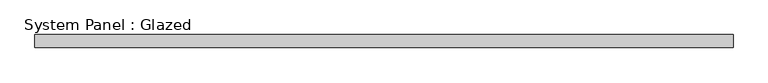
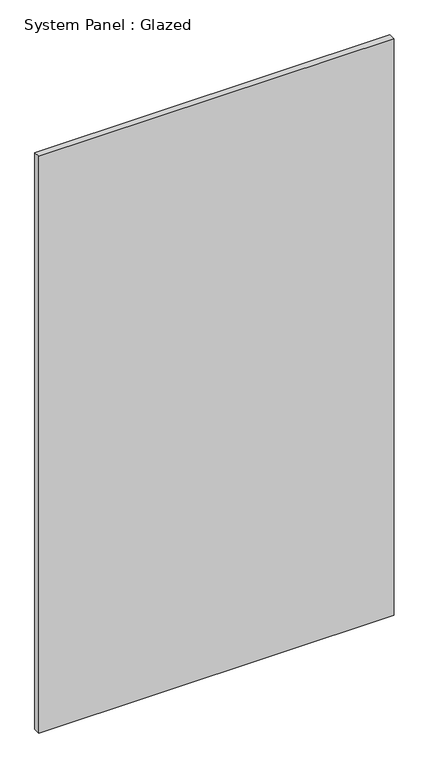
"""IFC4 building model written with IfcOpenShell, lengths in millimetres: plate geometry, System Panel : Glazed."""

from ifc_helpers import new_model, si_unit, origin, origin_with_axes, place, context, project, spatial, polyline, outline, extrude, source, transform, mapped, element, save


def system_panel_glazed_660e552d(model_context):
    return source(origin(), model_context, "Body", "SweptSolid", [
        extrude(outline(polyline([(683.0342567, 19.05), (-683.0342567, 19.05), (-683.0342567, 44.45), (683.0342567, 44.45), (683.0342567, 19.05)])), origin_with_axes(), (0.0, 0.0, 1.0), 2343.15),
    ])


if __name__ == "__main__":
    model = new_model("IFC4")
    model_context = context("Model", 3, world=origin())
    ifc_project = project(units=[si_unit("LENGTHUNIT", "METRE", prefix="MILLI")], contexts=[model_context])
    site = spatial("IfcSite", under=ifc_project)
    building = spatial("IfcBuilding", under=site)
    placement = place(None, origin())
    system_panel_glazed_shape = system_panel_glazed_660e552d(model_context)
    element("IfcPlate", 1, ObjectType="System Panel : Glazed", at=placement, inside=building, context=model_context, shape_type="MappedRepresentation", body=[
        mapped(system_panel_glazed_shape, transform((0.0, 0.0, 0.0), x_axis=(1.0, 0.0, 0.0), y_axis=(0.0, 1.0, 0.0), z_axis=(0.0, 0.0, 1.0))),
    ])
    save(model, "model.ifc")

# Revit data of these elements
# Type "System Panel : Glazed"
#   Construction Type Id = "GSP4R"
#   Analytic Construction = "1/8 in Pilkington single glazing"
#   Visual Light Transmittance = 0.9
#   Solar Heat Gain Coefficient = 0.86
#   Heat Transfer Coefficient (U) = 1.18115 BTU/(h·ft²·°F)
# Element 1 (IfcPlate, "System Panel : Glazed")
#   Materials on its faces: "Glass"
# Materials
#   "Glass": class "Glass", colour RGB 0 128 192, transparency 0.75, Description = "Soda Lime Glass", Cost = 0
